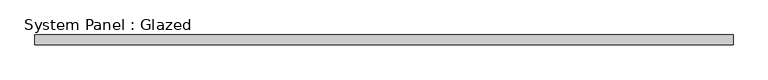
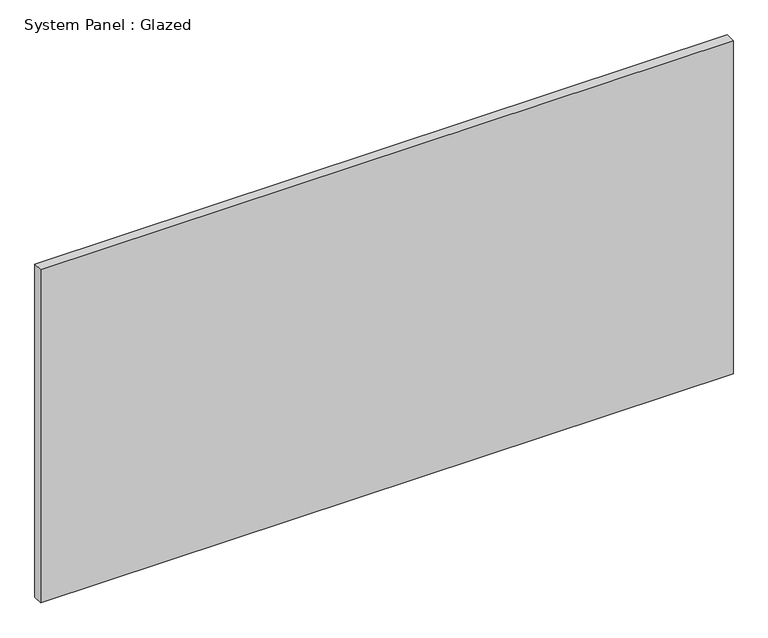
"""IFC4 building model written with IfcOpenShell, lengths in millimetres: plate geometry, System Panel : Glazed."""

from ifc_helpers import new_model, si_unit, origin, origin_with_axes, place, context, project, spatial, polyline, outline, extrude, source, transform, mapped, element, save


def system_panel_glazed_0021da76(model_context):
    return source(origin(), model_context, "Body", "SweptSolid", [
        extrude(outline(polyline([(882.65, 19.05), (-882.65, 19.05), (-882.65, 44.45), (882.65, 44.45), (882.65, 19.05)])), origin_with_axes(), (0.0, 0.0, 1.0), 897.5064813),
    ])


if __name__ == "__main__":
    model = new_model("IFC4")
    model_context = context("Model", 3, world=origin())
    ifc_project = project(units=[si_unit("LENGTHUNIT", "METRE", prefix="MILLI")], contexts=[model_context])
    site = spatial("IfcSite", under=ifc_project)
    building = spatial("IfcBuilding", under=site)
    placement = place(None, origin())
    system_panel_glazed_shape = system_panel_glazed_0021da76(model_context)
    element("IfcPlate", 1, ObjectType="System Panel : Glazed", at=placement, inside=building, context=model_context, shape_type="MappedRepresentation", body=[
        mapped(system_panel_glazed_shape, transform((0.0, 0.0, 0.0), x_axis=(1.0, 0.0, 0.0), y_axis=(0.0, 1.0, 0.0), z_axis=(0.0, 0.0, 1.0))),
    ])
    save(model, "model.ifc")

# Revit data of these elements
# Type "System Panel : Glazed"
#   Construction Type Id = "GSP4R"
#   Analytic Construction = "1/8 in Pilkington single glazing"
#   Visual Light Transmittance = 0.9
#   Solar Heat Gain Coefficient = 0.86
#   Heat Transfer Coefficient (U) = 1.18115 BTU/(h·ft²·°F)
#   Define Thermal Properties by = 1
# Element 1 (IfcPlate, "System Panel : Glazed")
#   Materials on its faces: "Glass"
# Materials
#   "Glass": class "Glass", colour RGB 0 128 192, transparency 0.75, Description = "Soda Lime Glass", Cost = 0
